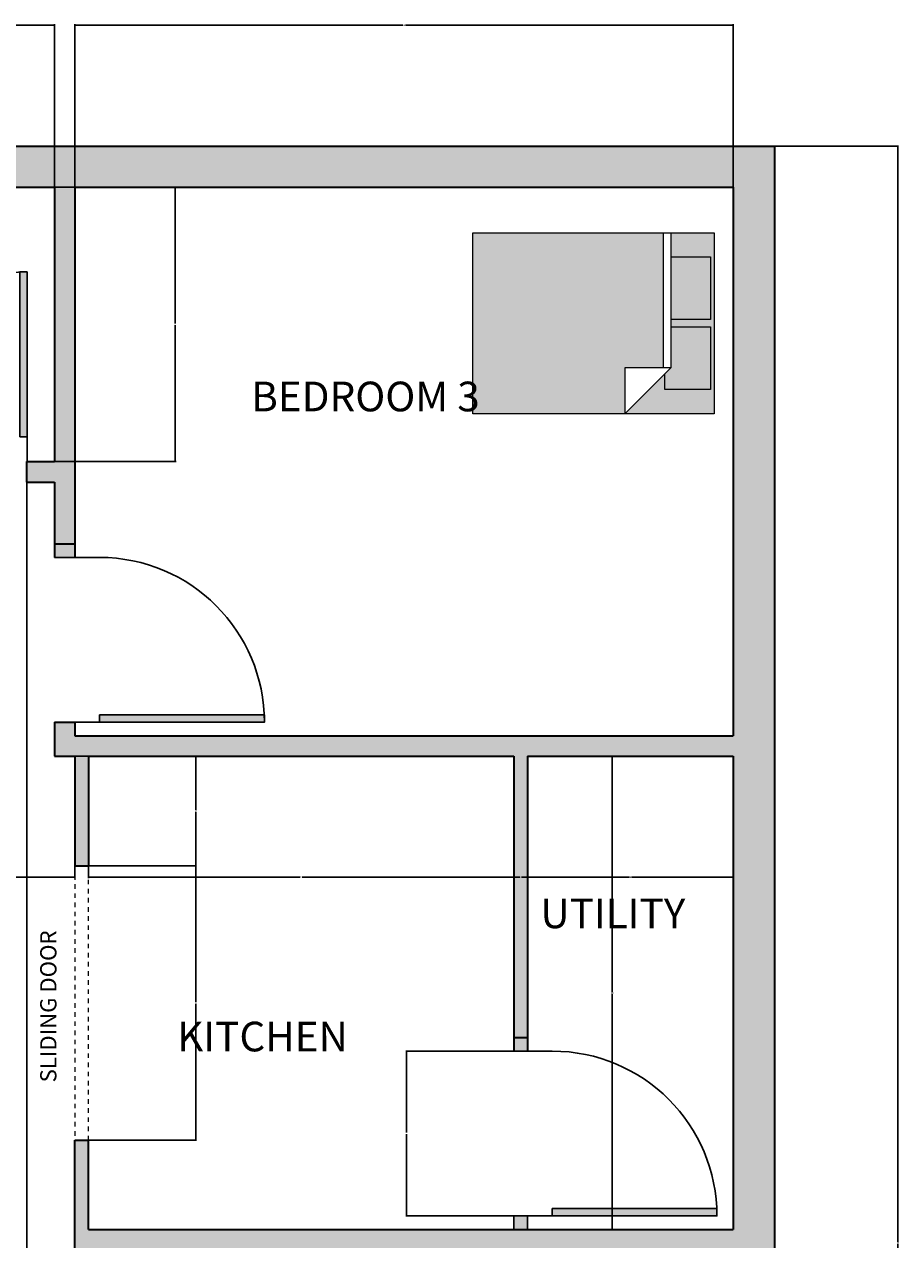
# Model space of a CAD drawing. Units: inches. Extents: x 1034 to 1730, y 674 to 1249.
# Tile 4 of 4: x 1538 to 1730, y 983 to 1249. Entities that reach past the tile are written whole.
import ezdxf

# ---------------------------------------------------------------- set-up
doc = ezdxf.new("R2010")
doc.units = ezdxf.units.IN
doc.linetypes.add('JIS_02_1.0', pattern=[2, 1, -1])
for name, color, linetype, lineweight in [('A-ANNO-DIMS', 2, 'Continuous', 18), ('A-ANNO-TEXT', 7, 'Continuous', 18), ('A-AREA-IDEN', 7, 'Continuous', 18), ('A-DOOR', 4, 'Continuous', 25), ('A-DOOR-HIDN', 4, 'JIS_02_1.0', 18), ('A-FURN', 9, 'Continuous', 18), ('A-FURN-PATT', 7, 'Continuous', 13), ('A-WALL', 7, 'Continuous', 35), ('A-WALL-PATT', 8, 'Continuous', 13)]:
    doc.layers.add(name, color=color, linetype=linetype, lineweight=lineweight)
doc.layers.add('A-DOOR-PATT', color=17, linetype='Continuous', lineweight=13, true_color=0x7b4636)
doc.styles.get("Standard").update_dxf_attribs({"font": 'arial.ttf'})
doc.dimstyles.get("Standard").update_dxf_attribs({"dimtxt": 0.18, "dimasz": 0.18, "dimexe": 0.18, "dimexo": 0.0625, "dimgap": 0.09, "dimtad": 0, "dimtih": 1, "dimtoh": 1, "dimdec": 4, "dimzin": 0, "dimdsep": 46, "dimtxsty": 'Standard', "dimcen": 0.09, "dimadec": 0, "dimazin": 0, "dimtfac": 1, "dimtdec": 4, "dimtofl": 0, "dimtmove": 0, "dimatfit": 3, "dimfxl": 1, "dimtolj": 1, "dimtzin": 0, "dimarcsym": 0})

# ---------------------------------------------------------------- blocks, each defined once
blk = doc.blocks.new('*U4')
for p, q in [((0, 0), (0, -6)), ((-40, 0), (-40, -6))]:
    blk.add_line(p, q)
blk.add_lwpolyline([(0, 0), (0, 40), (-1.75, 40), (-1.75, 0)], close=True)
blk.add_arc((0, 0), 40, 90, 180)
blk = doc.blocks.new('*U5')
for p, q in [((0, 0), (0, -6)), ((-40, 0), (-40, -6))]:
    blk.add_line(p, q)
blk.add_lwpolyline([(0, 0), (0, 40), (-1.75, 40), (-1.75, 0)], close=True)
blk.add_arc((0, 0), 40, 90, 180)
blk = doc.blocks.new('Bed - Queen')
for p, q in [((0, -80.00003), (0, 0)), ((0, 0), (59.99999, 0)), ((59.99999, 0), (59.99999, -80.00003)), ((7.99999, -1.2), (28.79998, -1.2)), ((7.99999, -14.4), (7.99999, -1.2)), ((28.79998, -1.2), (28.79998, -14.4)), ((31.19999, -1.2), (51.99999, -1.2)), ((31.19999, -14.4), (31.19999, -1.2)), ((51.99999, -1.2), (51.99999, -16.4)), ((0, -14.4), (44.8, -14.4)), ((59.99999, -29.6), (44.8, -14.4)), ((44.8, -14.4), (44.8, -29.6)), ((44.8, -16.8), (0, -16.8)), ((51.99999, -16.4), (46.79936, -16.4)), ((44.8, -29.6), (59.99999, -29.6)), ((59.99999, -80.00003), (0, -80.00003))]:
    blk.add_line(p, q)
blk = doc.blocks.new('*D15')
at = {"layer": 'A-ANNO-DIMS', "color": 0, "lineweight": -2, "transparency": 16777216}
for p, q in [((1702.59, 1222.43), (1729.69, 1222.43)), ((1729.51, 1222.25), (1729.51, 982.61)), ((1729.51, 742.61), (1729.51, 982.24)), ((1702.59, 742.43), (1729.69, 742.43))]:
    blk.add_line(p, q, dxfattribs=at)
at = {"layer": 'A-ANNO-DIMS', "color": 0, "transparency": 16777216}
for points in [[(1729.48, 1222.25), (1729.54, 1222.25), (1729.51, 1222.43)], [(1729.48, 742.61), (1729.54, 742.61), (1729.51, 742.43)]]:
    blk.add_solid(points, dxfattribs=at)
at = {"layer": 'Defpoints', "color": 0, "transparency": 16777216}
for p in [(1702.53, 1222.43), (1729.51, 1222.43), (1702.53, 742.43)]:
    blk.add_point(p, dxfattribs=at)
at = {"layer": 'A-ANNO-DIMS', "color": 0, "transparency": 16777216, "insert": (1729.51, 982.43), "char_height": 0.18, "attachment_point": 5}
blk.add_mtext('\\A1;480', dxfattribs=at)
blk = doc.blocks.new('*D18')
at = {"layer": 'A-ANNO-DIMS', "color": 0, "lineweight": -2, "transparency": 16777216}
for p, q in [((1549.53, 1213.49), (1549.53, 1249.06)), ((1549.71, 1248.88), (1621.25, 1248.88)), ((1693.35, 1248.88), (1621.81, 1248.88)), ((1693.53, 1213.49), (1693.53, 1249.06))]:
    blk.add_line(p, q, dxfattribs=at)
at = {"layer": 'A-ANNO-DIMS', "color": 0, "transparency": 16777216}
for points in [[(1549.71, 1248.91), (1549.71, 1248.85), (1549.53, 1248.88)], [(1693.35, 1248.91), (1693.35, 1248.85), (1693.53, 1248.88)]]:
    blk.add_solid(points, dxfattribs=at)
at = {"layer": 'Defpoints', "color": 0, "transparency": 16777216}
for p in [(1693.53, 1248.88), (1549.53, 1213.43), (1693.53, 1213.43)]:
    blk.add_point(p, dxfattribs=at)
at = {"layer": 'A-ANNO-DIMS', "color": 0, "transparency": 16777216, "insert": (1621.53, 1248.88), "char_height": 0.18, "attachment_point": 5}
blk.add_mtext('\\A1;144', dxfattribs=at)
blk = doc.blocks.new('*D26')
at = {"layer": 'A-ANNO-DIMS', "color": 0, "lineweight": -2, "transparency": 16777216}
for p, q in [((1500.03, 1213.49), (1500.03, 1249.06)), ((1500.21, 1248.88), (1522.31, 1248.88)), ((1544.85, 1248.88), (1522.75, 1248.88)), ((1545.03, 1213.49), (1545.03, 1249.06))]:
    blk.add_line(p, q, dxfattribs=at)
at = {"layer": 'A-ANNO-DIMS', "color": 0, "transparency": 16777216}
for points in [[(1500.21, 1248.91), (1500.21, 1248.85), (1500.03, 1248.88)], [(1544.85, 1248.91), (1544.85, 1248.85), (1545.03, 1248.88)]]:
    blk.add_solid(points, dxfattribs=at)
at = {"layer": 'Defpoints', "color": 0, "transparency": 16777216}
for p in [(1545.03, 1248.88), (1500.03, 1213.43), (1545.03, 1213.43)]:
    blk.add_point(p, dxfattribs=at)
at = {"layer": 'A-ANNO-DIMS', "color": 0, "transparency": 16777216, "insert": (1522.53, 1248.88), "char_height": 0.18, "attachment_point": 5}
blk.add_mtext('\\A1;45', dxfattribs=at)
blk = doc.blocks.new('*D27')
at = {"layer": 'A-ANNO-DIMS', "color": 0, "lineweight": -2, "transparency": 16777216}
for p, q in [((1545.09, 1213.43), (1571.66, 1213.43)), ((1571.48, 1213.25), (1571.48, 1183.61)), ((1571.48, 1153.61), (1571.48, 1183.24)), ((1545.09, 1153.43), (1571.66, 1153.43))]:
    blk.add_line(p, q, dxfattribs=at)
at = {"layer": 'A-ANNO-DIMS', "color": 0, "transparency": 16777216}
for points in [[(1571.45, 1213.25), (1571.51, 1213.25), (1571.48, 1213.43)], [(1571.45, 1153.61), (1571.51, 1153.61), (1571.48, 1153.43)]]:
    blk.add_solid(points, dxfattribs=at)
at = {"layer": 'Defpoints', "color": 0, "transparency": 16777216}
for p in [(1545.03, 1213.43), (1545.03, 1153.43), (1571.48, 1153.43)]:
    blk.add_point(p, dxfattribs=at)
at = {"layer": 'A-ANNO-DIMS', "color": 0, "transparency": 16777216, "insert": (1571.48, 1183.43), "char_height": 0.18, "attachment_point": 5}
blk.add_mtext('\\A1;60', dxfattribs=at)
blk = doc.blocks.new('*D28')
at = {"layer": 'A-ANNO-DIMS', "color": 0, "lineweight": -2, "transparency": 16777216}
for p, q in [((1503.03, 1153.36), (1503.03, 673.53)), ((1539.03, 1153.36), (1539.03, 673.53)), ((1503.21, 673.71), (1520.81, 673.71)), ((1538.85, 673.71), (1521.25, 673.71))]:
    blk.add_line(p, q, dxfattribs=at)
at = {"layer": 'A-ANNO-DIMS', "color": 0, "transparency": 16777216}
for points in [[(1503.21, 673.74), (1503.21, 673.68), (1503.03, 673.71)], [(1538.85, 673.74), (1538.85, 673.68), (1539.03, 673.71)]]:
    blk.add_solid(points, dxfattribs=at)
at = {"layer": 'Defpoints', "color": 0, "transparency": 16777216}
for p in [(1503.03, 1153.43), (1539.03, 1153.43), (1539.03, 673.71)]:
    blk.add_point(p, dxfattribs=at)
at = {"layer": 'A-ANNO-DIMS', "color": 0, "transparency": 16777216, "insert": (1521.03, 673.71), "char_height": 0.18, "attachment_point": 5}
blk.add_mtext('\\A1;36', dxfattribs=at)
blk = doc.blocks.new('*D33')
at = {"layer": 'A-ANNO-DIMS', "color": 0, "lineweight": -2, "transparency": 16777216}
for p, q in [((1552.53, 1088.86), (1552.53, 1062.3)), ((1645.53, 1088.86), (1645.53, 1062.3)), ((1552.71, 1062.48), (1598.81, 1062.48)), ((1645.35, 1062.48), (1599.25, 1062.48))]:
    blk.add_line(p, q, dxfattribs=at)
at = {"layer": 'A-ANNO-DIMS', "color": 0, "transparency": 16777216}
for points in [[(1552.71, 1062.51), (1552.71, 1062.45), (1552.53, 1062.48)], [(1645.35, 1062.51), (1645.35, 1062.45), (1645.53, 1062.48)]]:
    blk.add_solid(points, dxfattribs=at)
at = {"layer": 'Defpoints', "color": 0, "transparency": 16777216}
for p in [(1552.53, 1088.93), (1645.53, 1088.93), (1552.53, 1062.48)]:
    blk.add_point(p, dxfattribs=at)
at = {"layer": 'A-ANNO-DIMS', "color": 0, "transparency": 16777216, "insert": (1599.03, 1062.48), "char_height": 0.18, "attachment_point": 5}
blk.add_mtext('\\A1;93', dxfattribs=at)
blk = doc.blocks.new('*D34')
at = {"layer": 'A-ANNO-DIMS', "color": 0, "lineweight": -2, "transparency": 16777216}
for p, q in [((1648.53, 1088.86), (1648.53, 1062.3)), ((1693.53, 1088.86), (1693.53, 1062.3)), ((1648.71, 1062.48), (1670.81, 1062.48)), ((1693.35, 1062.48), (1671.25, 1062.48))]:
    blk.add_line(p, q, dxfattribs=at)
at = {"layer": 'A-ANNO-DIMS', "color": 0, "transparency": 16777216}
for points in [[(1648.71, 1062.51), (1648.71, 1062.45), (1648.53, 1062.48)], [(1693.35, 1062.51), (1693.35, 1062.45), (1693.53, 1062.48)]]:
    blk.add_solid(points, dxfattribs=at)
at = {"layer": 'Defpoints', "color": 0, "transparency": 16777216}
for p in [(1648.53, 1088.93), (1693.53, 1088.93), (1648.53, 1062.48)]:
    blk.add_point(p, dxfattribs=at)
at = {"layer": 'A-ANNO-DIMS', "color": 0, "transparency": 16777216, "insert": (1671.03, 1062.48), "char_height": 0.18, "attachment_point": 5}
blk.add_mtext('\\A1;45', dxfattribs=at)
blk = doc.blocks.new('*D35')
at = {"layer": 'A-ANNO-DIMS', "color": 0, "lineweight": -2, "transparency": 16777216}
for p, q in [((1693.47, 1088.93), (1666.9, 1088.93)), ((1667.08, 1088.75), (1667.08, 1037.36)), ((1667.08, 985.61), (1667.08, 1036.99)), ((1693.47, 985.43), (1666.9, 985.43))]:
    blk.add_line(p, q, dxfattribs=at)
at = {"layer": 'A-ANNO-DIMS', "color": 0, "transparency": 16777216}
for points in [[(1667.05, 1088.75), (1667.11, 1088.75), (1667.08, 1088.93)], [(1667.05, 985.61), (1667.11, 985.61), (1667.08, 985.43)]]:
    blk.add_solid(points, dxfattribs=at)
at = {"layer": 'Defpoints', "color": 0, "transparency": 16777216}
for p in [(1667.08, 1088.93), (1693.53, 1088.93), (1693.53, 985.43)]:
    blk.add_point(p, dxfattribs=at)
at = {"layer": 'A-ANNO-DIMS', "color": 0, "transparency": 16777216, "insert": (1667.08, 1037.18), "char_height": 0.18, "attachment_point": 5}
blk.add_mtext('\\A1;103.5', dxfattribs=at)
blk = doc.blocks.new('*D36')
at = {"layer": 'A-ANNO-DIMS', "color": 0, "lineweight": -2, "transparency": 16777216}
for p, q in [((1549.59, 1064.93), (1576.16, 1064.93)), ((1575.98, 1064.75), (1575.98, 1035.11)), ((1575.98, 1005.11), (1575.98, 1034.74)), ((1549.59, 1004.93), (1576.16, 1004.93))]:
    blk.add_line(p, q, dxfattribs=at)
at = {"layer": 'A-ANNO-DIMS', "color": 0, "transparency": 16777216}
for points in [[(1575.95, 1064.75), (1576.01, 1064.75), (1575.98, 1064.93)], [(1575.95, 1005.11), (1576.01, 1005.11), (1575.98, 1004.93)]]:
    blk.add_solid(points, dxfattribs=at)
at = {"layer": 'Defpoints', "color": 0, "transparency": 16777216}
for p in [(1549.53, 1064.93), (1549.53, 1004.93), (1575.98, 1004.93)]:
    blk.add_point(p, dxfattribs=at)
at = {"layer": 'A-ANNO-DIMS', "color": 0, "transparency": 16777216, "insert": (1575.98, 1034.93), "char_height": 0.18, "attachment_point": 5}
blk.add_mtext('\\A1;60', dxfattribs=at)
blk = doc.blocks.new('*D37')
at = {"layer": 'A-ANNO-DIMS', "color": 0, "lineweight": -2, "transparency": 16777216}
for p, q in [((1549.59, 1088.93), (1576.16, 1088.93)), ((1575.98, 1088.75), (1575.98, 1077.11)), ((1575.98, 1065.11), (1575.98, 1076.75)), ((1549.59, 1064.93), (1576.16, 1064.93))]:
    blk.add_line(p, q, dxfattribs=at)
at = {"layer": 'A-ANNO-DIMS', "color": 0, "transparency": 16777216}
for points in [[(1575.95, 1088.75), (1576.01, 1088.75), (1575.98, 1088.93)], [(1575.95, 1065.11), (1576.01, 1065.11), (1575.98, 1064.93)]]:
    blk.add_solid(points, dxfattribs=at)
at = {"layer": 'Defpoints', "color": 0, "transparency": 16777216}
for p in [(1549.53, 1088.93), (1549.53, 1064.93), (1575.98, 1064.93)]:
    blk.add_point(p, dxfattribs=at)
at = {"layer": 'A-ANNO-DIMS', "color": 0, "transparency": 16777216, "insert": (1575.98, 1076.93), "char_height": 0.18, "attachment_point": 5}
blk.add_mtext('\\A1;24', dxfattribs=at)
blk = doc.blocks.new('*D38')
at = {"layer": 'A-ANNO-DIMS', "color": 0, "lineweight": -2, "transparency": 16777216}
for p, q in [((1648.47, 1024.43), (1621.9, 1024.43)), ((1622.08, 1024.25), (1622.08, 1006.61)), ((1622.08, 988.61), (1622.08, 1006.24)), ((1648.47, 988.43), (1621.9, 988.43))]:
    blk.add_line(p, q, dxfattribs=at)
at = {"layer": 'A-ANNO-DIMS', "color": 0, "transparency": 16777216}
for points in [[(1622.05, 1024.25), (1622.11, 1024.25), (1622.08, 1024.43)], [(1622.05, 988.61), (1622.11, 988.61), (1622.08, 988.43)]]:
    blk.add_solid(points, dxfattribs=at)
at = {"layer": 'Defpoints', "color": 0, "transparency": 16777216}
for p in [(1622.08, 1024.43), (1648.53, 1024.43), (1648.53, 988.43)]:
    blk.add_point(p, dxfattribs=at)
at = {"layer": 'A-ANNO-DIMS', "color": 0, "transparency": 16777216, "insert": (1622.08, 1006.43), "char_height": 0.18, "attachment_point": 5}
blk.add_mtext('\\A1;36', dxfattribs=at)
blk = doc.blocks.new('*D42')
at = {"layer": 'A-ANNO-DIMS', "color": 0, "lineweight": -2, "transparency": 16777216}
for p, q in [((1645.53, 1088.86), (1645.53, 1062.3)), ((1648.53, 1088.86), (1648.53, 1062.3)), ((1645.71, 1062.48), (1646.88, 1062.48)), ((1648.35, 1062.48), (1647.18, 1062.48))]:
    blk.add_line(p, q, dxfattribs=at)
at = {"layer": 'A-ANNO-DIMS', "color": 0, "transparency": 16777216}
for points in [[(1645.71, 1062.51), (1645.71, 1062.45), (1645.53, 1062.48)], [(1648.35, 1062.51), (1648.35, 1062.45), (1648.53, 1062.48)]]:
    blk.add_solid(points, dxfattribs=at)
at = {"layer": 'Defpoints', "color": 0, "transparency": 16777216}
for p in [(1645.53, 1088.93), (1648.53, 1088.93), (1645.53, 1062.48)]:
    blk.add_point(p, dxfattribs=at)
at = {"layer": 'A-ANNO-DIMS', "color": 0, "transparency": 16777216, "insert": (1647.03, 1062.48), "char_height": 0.18, "attachment_point": 5}
blk.add_mtext('\\A1;3', dxfattribs=at)
blk = doc.blocks.new('*D46')
at = {"layer": 'A-ANNO-DIMS', "color": 0, "lineweight": -2, "transparency": 16777216}
for p, q in [((1351.53, 1088.86), (1351.53, 1062.3)), ((1549.53, 1088.86), (1549.53, 1062.3)), ((1351.71, 1062.48), (1450.25, 1062.48)), ((1549.35, 1062.48), (1450.81, 1062.48))]:
    blk.add_line(p, q, dxfattribs=at)
at = {"layer": 'A-ANNO-DIMS', "color": 0, "transparency": 16777216}
for points in [[(1351.71, 1062.51), (1351.71, 1062.45), (1351.53, 1062.48)], [(1549.35, 1062.51), (1549.35, 1062.45), (1549.53, 1062.48)]]:
    blk.add_solid(points, dxfattribs=at)
at = {"layer": 'Defpoints', "color": 0, "transparency": 16777216}
for p in [(1351.53, 1088.93), (1549.53, 1088.93), (1351.53, 1062.48)]:
    blk.add_point(p, dxfattribs=at)
at = {"layer": 'A-ANNO-DIMS', "color": 0, "transparency": 16777216, "insert": (1450.53, 1062.48), "char_height": 0.18, "attachment_point": 5}
blk.add_mtext('\\A1;198', dxfattribs=at)

msp = doc.modelspace()

# ---------------------------------------------------------------- hatches: boundary and pattern name
at = {"layer": 'A-DOOR-PATT'}
h = msp.add_hatch(color=256, dxfattribs=at)
h.dxf.hatch_style = 1
h.paths.add_polyline_path([(1490.123, 922.4262), (1454.0839, 922.4262, 0.01094143), (1454.1184, 920.8495), (1490.123, 920.8495)])
h.paths.add_polyline_path([(1540.7238, 871.4262), (1504.6847, 871.4262), (1504.6847, 869.8495), (1540.6893, 869.8495, 0.01094143)])
h.paths.add_polyline_path([(1503.0288, 874.4262), (1495.5288, 874.4262), (1495.5288, 871.4262), (1503.0288, 871.4262)])
h.paths.add_polyline_path([(1503.0288, 835.3871), (1499.2788, 835.3871), (1495.5288, 835.4262), (1495.5288, 832.4262), (1503.0288, 832.4262)])
h.paths.add_polyline_path([(1564.6056, 873.3367, 0.01094143), (1563.0288, 873.3712), (1563.0288, 837.3321), (1564.6056, 837.3321)])
h.paths.add_polyline_path([(1602.0288, 831.9262), (1599.0288, 831.9262), (1599.0288, 828.9262), (1602.0288, 828.9262)])
h.paths.add_polyline_path([(1648.5288, 988.4262), (1645.5288, 988.4262), (1645.5288, 985.4262), (1648.5288, 985.4262)])
h.paths.add_polyline_path([(1689.9738, 989.9638), (1653.9347, 989.9638), (1653.9347, 988.3871), (1689.9738, 988.3871)])
h.paths.add_polyline_path([(1648.5288, 1027.4262), (1645.5288, 1027.4262), (1645.5288, 1024.4262), (1648.5288, 1024.4262)])
h.paths.add_polyline_path([(1590.9393, 1097.9638), (1554.9347, 1097.9638), (1554.9347, 1096.3871), (1590.9738, 1096.3871, 0.01094143)])
h.paths.add_polyline_path([(1549.5288, 1135.4262), (1545.0288, 1135.4262), (1545.0288, 1132.4262), (1549.5288, 1132.4262)])
h.paths.add_polyline_path([(1500.0288, 1135.4262), (1495.5288, 1135.4262), (1495.5288, 1132.4262), (1500.0288, 1132.4262)])
h.paths.add_polyline_path([(1490.123, 1098.0029), (1454.0839, 1098.0029), (1454.0839, 1096.4262), (1490.123, 1096.4262)])
h.paths.add_polyline_path([(1539.068, 1194.8712, 0.01094143), (1537.4912, 1194.8367), (1537.4912, 1158.8321), (1539.068, 1158.8321)])
at = {"layer": 'A-FURN-PATT'}
h = msp.add_hatch(color=256, dxfattribs=at)
h.dxf.hatch_style = 1
h.paths.add_polyline_path([(1414.278, 838.2731), (1381.0078, 838.2731), (1381.0078, 828.2392), (1372.5582, 828.2392), (1372.5582, 798.6657), (1414.278, 798.6657)])
h.paths.add_polyline_path([(1370.9739, 828.2392), (1372.2941, 829.5594), (1372.2941, 832.9921), (1362.2603, 832.9921), (1362.2603, 819.2615), (1370.9739, 819.2615)], flags=17)
h.paths.add_polyline_path([(1370.9739, 817.6772), (1362.2603, 817.6772), (1362.2603, 803.9467), (1370.9739, 803.9467)], flags=17)
h.paths.add_polyline_path([(1367.0568, 1198.6055), (1368.377, 1199.9257), (1368.377, 1203.3584), (1358.3431, 1203.3584), (1358.3431, 1189.6278), (1367.0568, 1189.6278)], flags=17)
h.paths.add_polyline_path([(1367.0568, 1188.0435), (1358.3431, 1188.0435), (1358.3431, 1174.3129), (1367.0568, 1174.3129)], flags=17)
h.paths.add_polyline_path([(1410.3609, 1208.6394), (1377.0906, 1208.6394), (1377.0906, 1198.6055), (1368.6411, 1198.6055), (1368.6411, 1169.032), (1410.3609, 1169.032)])
h.paths.add_polyline_path([(1678.2824, 1203.4604), (1636.5626, 1203.4604), (1636.5626, 1163.853), (1669.8329, 1163.853), (1669.8329, 1173.8868), (1678.2824, 1173.8868)])
h.paths.add_polyline_path([(1688.5804, 1182.8645), (1679.8667, 1182.8645), (1679.8667, 1173.8868), (1678.5465, 1172.5666), (1678.5465, 1169.1339), (1688.5804, 1169.1339)], flags=17)
h.paths.add_polyline_path([(1367.0568, 1174.3129), (1358.3431, 1174.3129), (1358.3431, 1188.0435), (1367.0568, 1188.0435), (1367.0568, 1189.6278), (1358.3431, 1189.6278), (1358.3431, 1203.3584), (1368.377, 1203.3584), (1368.377, 1199.9257), (1377.0906, 1208.6394), (1357.551, 1208.6394), (1357.551, 1169.032), (1367.0568, 1169.032)])
h.paths.add_polyline_path([(1688.5804, 1198.1794), (1679.8667, 1198.1794), (1679.8667, 1184.4488), (1688.5804, 1184.4488)], flags=17)
h.paths.add_polyline_path([(1689.3725, 1203.4604), (1679.8667, 1203.4604), (1679.8667, 1198.1794), (1688.5804, 1198.1794), (1688.5804, 1184.4488), (1679.8667, 1184.4488), (1679.8667, 1182.8645), (1688.5804, 1182.8645), (1688.5804, 1169.1339), (1678.5465, 1169.1339), (1678.5465, 1172.5666), (1669.8329, 1163.853), (1689.3725, 1163.853)])
h.paths.add_polyline_path([(1370.9739, 803.9467), (1362.2603, 803.9467), (1362.2603, 817.6772), (1370.9739, 817.6772), (1370.9739, 819.2615), (1362.2603, 819.2615), (1362.2603, 832.9921), (1372.2941, 832.9921), (1372.2941, 829.5594), (1381.0078, 838.2731), (1361.4681, 838.2731), (1361.4681, 798.6657), (1370.9739, 798.6657)])
h.paths.add_polyline_path([(1586.4252, 1162.5974), (1646.7165, 1162.5974), (1646.7165, 1172.6784), (1586.4252, 1172.6784)], flags=9)
h.paths.add_polyline_path([(1574.2942, 863.9077), (1611.4062, 863.9077), (1611.4062, 873.9821), (1574.2942, 873.9821)], flags=9)
h.paths.add_polyline_path([(1502.8652, 818.6383), (1550.5629, 818.6383), (1550.5629, 828.7127), (1502.8652, 828.7127)], flags=9)
h.paths.add_polyline_path([(1367.7365, 861.2327), (1425.5064, 861.2327), (1425.5064, 871.3071), (1367.7365, 871.3071)], flags=9)
h.paths.add_polyline_path([(1409.7909, 1010.2859), (1487.2071, 1010.2859), (1487.2071, 1020.3537), (1409.7909, 1020.3537)], flags=9)
h.paths.add_polyline_path([(1499.9637, 1199.6865), (1545.1423, 1199.6865), (1545.1423, 1209.7608), (1499.9637, 1209.7608)], flags=9)
h.paths.add_polyline_path([(1378.5639, 1158.2313), (1436.3338, 1158.2313), (1436.3338, 1168.3057), (1378.5639, 1168.3057)], flags=9)
at = {"layer": 'A-WALL-PATT'}
h = msp.add_hatch(color=256, dxfattribs=at)
h.dxf.hatch_style = 1
h.paths.add_polyline_path([(1351.5288, 1213.4262), (1495.5288, 1213.4262), (1495.5288, 1135.4262), (1500.0288, 1135.4262), (1500.0288, 1148.9262), (1503.0288, 1148.9262), (1503.0288, 1153.4262), (1500.0288, 1153.4262), (1500.0288, 1213.4262), (1545.0288, 1213.4262), (1545.0288, 1153.4262), (1539.0288, 1153.4262), (1539.0288, 1148.9262), (1545.0288, 1148.9262), (1545.0288, 1135.4262), (1549.5288, 1135.4262), (1549.5288, 1213.4262), (1693.5288, 1213.4262), (1693.5288, 1093.4262), (1549.5288, 1093.4262), (1549.5288, 1096.4262), (1545.0288, 1096.4262), (1545.0288, 1088.9262), (1549.5288, 1088.9262), (1549.5288, 1064.9262), (1552.5288, 1064.9262), (1552.5288, 1088.9262), (1645.5288, 1088.9262), (1645.5288, 1027.4262), (1648.5288, 1027.4262), (1648.5288, 1088.9262), (1693.5288, 1088.9262), (1693.5288, 985.4262), (1552.5288, 985.4262), (1552.5288, 1004.9262), (1549.5288, 1004.9262), (1549.5288, 980.9262), (1620.0288, 980.9262), (1620.0288, 831.9262), (1602.0288, 831.9262), (1602.0288, 828.9262), (1624.5288, 828.9262), (1624.5288, 980.9262), (1693.5288, 980.9262), (1693.5288, 742.4262), (1702.5288, 742.4262), (1702.5288, 1222.4262), (1342.5288, 1222.4262), (1342.5288, 742.4262), (1620.0288, 742.4262), (1620.0288, 751.4262), (1351.5288, 751.4262), (1351.5288, 788.9262), (1560.0288, 788.9262), (1560.0288, 828.9262), (1563.0288, 828.9262), (1563.0288, 831.9262), (1560.0288, 831.9262), (1560.0288, 886.4262), (1500.0288, 886.4262), (1495.5288, 886.4262), (1495.5288, 874.4262), (1503.0288, 874.4262), (1503.0288, 883.4262), (1557.0288, 883.4262), (1557.0288, 791.9262), (1503.0288, 791.9262), (1503.0288, 832.4262), (1495.5288, 832.4262), (1495.5288, 793.4262), (1351.5288, 793.4262), (1351.5288, 925.4262), (1495.5288, 925.4262), (1495.5288, 922.4262), (1500.0288, 922.4262), (1500.0288, 929.9262), (1351.5288, 929.9262), (1351.5288, 1088.9262), (1500.0288, 1088.9262), (1500.0288, 1096.4262), (1495.5288, 1096.4262), (1495.5288, 1093.4262), (1351.5288, 1093.4262)])

# ---------------------------------------------------------------- linework, layer by layer
at = {"layer": 'A-DOOR'}
for p, q in [((1545.0288, 1132.4262), (1549.5288, 1132.4262)), ((1645.5288, 1024.4262), (1648.5288, 1024.4262)), ((1645.5288, 988.4262), (1648.5288, 988.4262)), ((1645.5288, 988.4262), (1645.5288, 985.4262)), ((1648.5288, 988.4262), (1648.5288, 985.4262))]:
    msp.add_line(p, q, dxfattribs=at)
at = {"layer": 'A-DOOR-HIDN'}
for p, q in [((1549.5288, 1064.9262), (1549.5288, 1004.9262)), ((1552.5288, 1004.9262), (1552.5288, 1064.9262))]:
    msp.add_line(p, q, dxfattribs=at)
at = {"layer": 'A-WALL'}
for p, q in [((1500.0288, 1213.4262), (1545.0288, 1213.4262)), ((1545.0288, 1213.4262), (1545.0288, 1153.4262)), ((1549.5288, 1213.4262), (1549.5288, 1132.4262)), ((1549.5288, 1213.4262), (1693.5288, 1213.4262)), ((1693.5288, 1213.4262), (1693.5288, 1093.4262)), ((1539.0288, 1148.9262), (1539.0288, 1153.4262)), ((1539.0288, 1153.4262), (1545.0288, 1153.4262)), ((1539.0288, 1148.9262), (1545.0288, 1148.9262)), ((1545.0288, 1148.9262), (1545.0288, 1132.4262)), ((1545.0288, 1135.4262), (1549.5288, 1135.4262)), ((1545.0288, 1096.4262), (1549.5288, 1096.4262)), ((1545.0288, 1096.4262), (1545.0288, 1088.9262)), ((1549.5288, 1096.4262), (1549.5288, 1093.4262)), ((1549.5288, 1093.4262), (1693.5288, 1093.4262)), ((1545.0288, 1088.9262), (1549.5288, 1088.9262)), ((1549.5288, 1088.9262), (1549.5288, 1064.9262)), ((1552.5288, 1088.9262), (1552.5288, 1064.9262)), ((1552.5288, 1088.9262), (1645.5288, 1088.9262)), ((1645.5288, 1088.9262), (1645.5288, 1024.4262)), ((1648.5288, 1088.9262), (1648.5288, 1024.4262)), ((1648.5288, 1088.9262), (1693.5288, 1088.9262)), ((1693.5288, 1088.9262), (1693.5288, 985.4262)), ((1549.5288, 1064.9262), (1552.5288, 1064.9262)), ((1645.5288, 1027.4262), (1648.5288, 1027.4262)), ((1549.5288, 980.9262), (1549.5288, 1004.9262)), ((1549.5288, 1004.9262), (1552.5288, 1004.9262)), ((1552.5288, 985.4262), (1552.5288, 1004.9262)), ((1552.5288, 985.4262), (1693.5288, 985.4262))]:
    msp.add_line(p, q, dxfattribs=at)
msp.add_lwpolyline([(1620.0288, 742.4262), (1342.5288, 742.4262), (1342.5288, 1222.4262), (1702.5288, 1222.4262), (1702.5288, 742.4262), (1693.5288, 742.4262)], dxfattribs=at)

# ---------------------------------------------------------------- block references
at = {"layer": 'A-DOOR', "xscale": 0.9009776753840846, "yscale": 0.9009776753840846, "zscale": 0.9009776753840846}
msp.add_blockref('*U5', (1539.068, 1158.8321), dxfattribs=at)
at = {"layer": 'A-DOOR', "xscale": 0.9009776753840846, "yscale": 0.9009776753840846, "zscale": 0.9009776753840846, "rotation": 270}
for p in [(1554.9347, 1096.3871), (1653.9347, 988.3871)]:
    msp.add_blockref('*U4', p, dxfattribs=at)
at = {"layer": 'A-FURN', "xscale": 0.6601233642522663, "yscale": 0.6601233642522663, "zscale": 0.6601233642522663, "rotation": 270}
msp.add_blockref('Bed - Queen', (1689.3725, 1203.4604), dxfattribs=at)

# ---------------------------------------------------------------- texts
at = {"layer": 'A-ANNO-TEXT'}
msp.add_text('SLIDING DOOR ', height=3.554228, rotation=90, dxfattribs=at).set_placement((1545.4886, 1017.5912))
at = {"layer": 'A-AREA-IDEN'}
for s, p in [('BEDROOM 3 ', (1588.1054, 1164.3927)), ('UTILITY ', (1651.3498, 1051.3238)), ('KITCHEN ', (1571.8945, 1024.3709))]:
    msp.add_text(s, height=6.49045, dxfattribs=at).set_placement(p)

# ---------------------------------------------------------------- dimensions: what is measured, and where the dimension line sits
at = {"layer": 'A-ANNO-DIMS'}
for base, p1, p2, picture, middle in [((1545.0288, 1248.8762), (1500.0288, 1213.4262), (1545.0288, 1213.4262), '*D26', (1522.5288, 1248.8762)), ((1693.5288, 1248.8762), (1549.5288, 1213.4262), (1693.5288, 1213.4262), '*D18', (1621.5288, 1248.8762)), ((1539.0288, 673.7132), (1503.0288, 1153.4262), (1539.0288, 1153.4262), '*D28', (1521.0288, 673.7132))]:
    dim = msp.add_linear_dim(base=base, p1=p1, p2=p2, dimstyle='Standard', override={"dimdec": 0, "dimlfac": 1, "dimrnd": 0, "dimzin": 0, "dimdsep": 46, "dimlunit": 2}, dxfattribs=at)
    dim.commit()
    dim.dimension.update_dxf_attribs({"geometry": picture, "text_midpoint": middle})
for base, p1, p2, angle, override, picture, middle in [((1729.5141, 1222.4262), (1702.5288, 742.4262), (1702.5288, 1222.4262), 90, {"dimdec": 0, "dimlfac": 1, "dimrnd": 0, "dimzin": 0, "dimdsep": 46, "dimlunit": 2}, '*D15', (1729.5141, 982.4262)), ((1571.4788, 1153.4262), (1545.0288, 1213.4262), (1545.0288, 1153.4262), 270, {"dimdec": 0, "dimlfac": 1, "dimrnd": 0, "dimzin": 0, "dimdsep": 46, "dimlunit": 2}, '*D27', (1571.4788, 1183.4262)), ((1351.5288, 1062.4762), (1549.5288, 1088.9262), (1351.5288, 1088.9262), 180, {"dimdec": 0, "dimlfac": 1, "dimrnd": 0, "dimzin": 0, "dimdsep": 46, "dimlunit": 2}, '*D46', (1450.5288, 1062.4762)), ((1575.9788, 1064.9262), (1549.5288, 1088.9262), (1549.5288, 1064.9262), 270, {"dimdec": 0, "dimlfac": 1, "dimrnd": 0, "dimzin": 0, "dimdsep": 46, "dimlunit": 2}, '*D37', (1575.9788, 1076.9262)), ((1552.5288, 1062.4762), (1645.5288, 1088.9262), (1552.5288, 1088.9262), 180, {"dimdec": 0, "dimlfac": 1, "dimrnd": 0, "dimzin": 0, "dimdsep": 46, "dimlunit": 2}, '*D33', (1599.0288, 1062.4762)), ((1645.5288, 1062.4762), (1648.5288, 1088.9262), (1645.5288, 1088.9262), 180, {"dimdec": 0, "dimlfac": 1, "dimrnd": 0, "dimzin": 0, "dimdsep": 46, "dimlunit": 2}, '*D42', (1647.0288, 1062.4762)), ((1648.5288, 1062.4762), (1693.5288, 1088.9262), (1648.5288, 1088.9262), 180, {"dimdec": 0, "dimlfac": 1, "dimrnd": 0, "dimzin": 0, "dimdsep": 46, "dimlunit": 2}, '*D34', (1671.0288, 1062.4762)), ((1667.0788, 1088.9262), (1693.5288, 985.4262), (1693.5288, 1088.9262), 90, {"dimdec": 1, "dimlfac": 1, "dimrnd": 0, "dimzin": 0, "dimdsep": 46, "dimlunit": 2}, '*D35', (1667.0788, 1037.1762)), ((1575.9788, 1004.9262), (1549.5288, 1064.9262), (1549.5288, 1004.9262), 270, {"dimdec": 0, "dimlfac": 1, "dimrnd": 0, "dimzin": 0, "dimdsep": 46, "dimlunit": 2}, '*D36', (1575.9788, 1034.9262)), ((1622.0788, 1024.4262), (1648.5288, 988.4262), (1648.5288, 1024.4262), 90, {"dimdec": 0, "dimlfac": 1, "dimrnd": 0, "dimzin": 0, "dimdsep": 46, "dimlunit": 2}, '*D38', (1622.0788, 1006.4262))]:
    dim = msp.add_linear_dim(base=base, p1=p1, p2=p2, angle=angle, dimstyle='Standard', override=override, dxfattribs=at)
    dim.commit()
    dim.dimension.update_dxf_attribs({"geometry": picture, "text_midpoint": middle})

doc.saveas('drawing.dxf')
